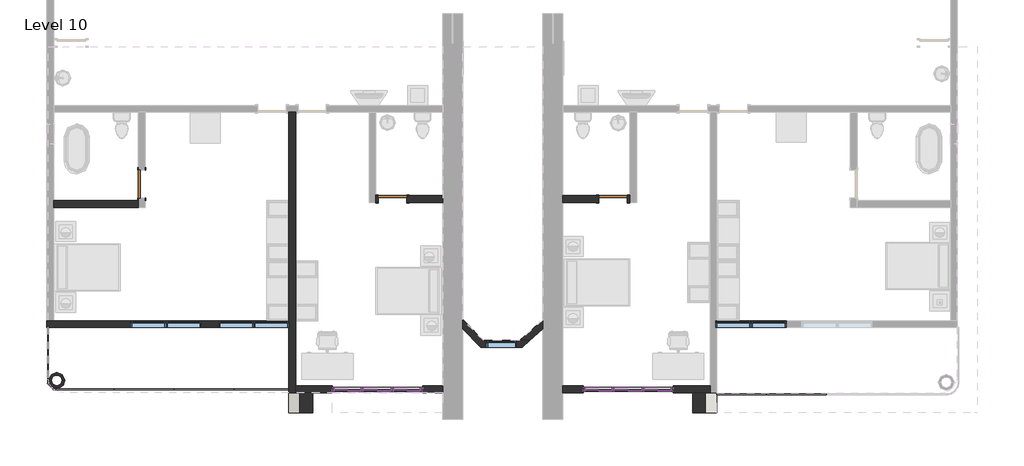
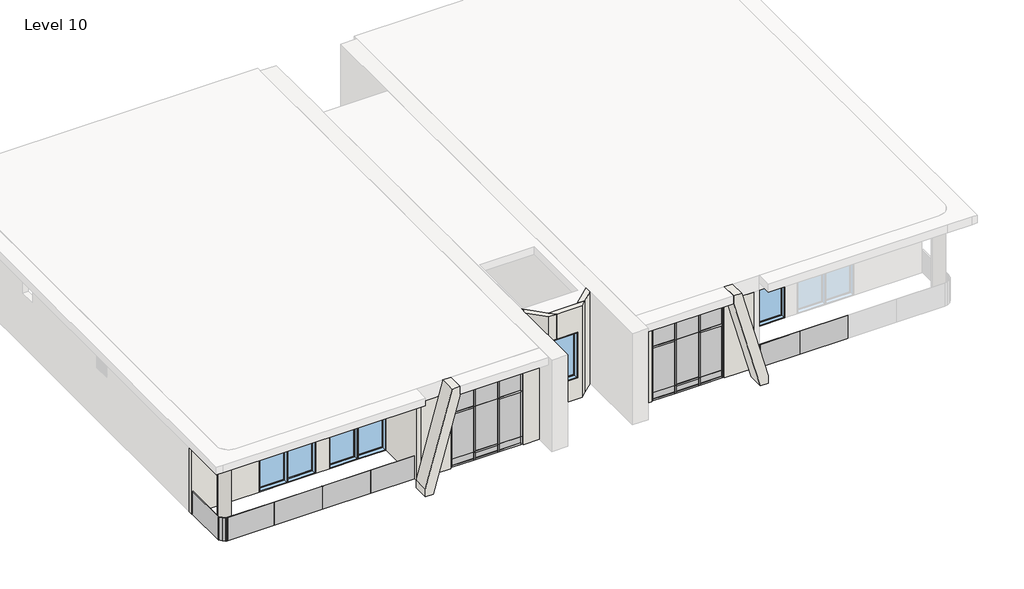
# One storey, part 1 of 3: 42 members, 29 plates, 16 walls, 7 windows, 3 doors.
"""IFC4 building model written with IfcOpenShell, lengths in millimetres."""

from ifc_helpers import new_model, si_unit, point, frame, frame_2d, origin, place, context, project, spatial, polyline, circle_curve, trimmed, segment, composite_curve, outline, extrude, faceted_brep, transform, mapped, element, save
from components import door_2703ae13, door_10fd3a06, member_c17f1be2, member_ad567e07, member_d2e7e466, member_7db1855a, member_75d1e245, member_d60e8053, member_3c3dc66a, member_2fae0574, member_410c6227, member_73c23c35, system_panel_glazed_38d54ecf, system_panel_glazed_fbb6c980, system_panel_glazed_4137532c, system_panel_glazed_6230de04, system_panel_glazed_a79f7f85, system_panel_glazed_9a5ea490, system_panel_glazed_95be5de7, system_panel_glazed_ffe51582, system_panel_glazed_8f95e3f6, system_panel_glazed_836907cd, system_panel_glazed_688a65a2, system_panel_glazed_c1a1c740, system_panel_glazed_22bcd51f, system_panel_glazed_524f965d, window_9a779fa2, window_1a213a25

model = new_model("IFC4")

# Units and contexts
model_context = context("Model", 3, world=origin())
ifc_project = project(units=[si_unit("LENGTHUNIT", "METRE", prefix="MILLI")], contexts=[model_context])

# Site, building, storey
site = spatial("IfcSite", under=ifc_project)
building = spatial("IfcBuilding", under=site)
storey = spatial("IfcBuildingStorey", under=building, Name="Level 10", Elevation=32918.4)

# Doors
placement = place(None, origin())
door_shape = door_2703ae13(model_context)
element("IfcDoor", 1, ObjectType="Door-Single-Panel.0001 : 34\" x 80\"", at=placement, inside=storey, context=model_context, shape_type="MappedRepresentation", body=[
    mapped(door_shape, transform((-15765.9987704, -441.9241442, 32918.4), x_axis=(0.0, -1.0, 0.0), y_axis=(1.0, 0.0, 0.0), z_axis=(0.0, 0.0, 1.0))),
])
element("IfcDoor", 2, ObjectType="Door-Single-Panel.0001 : 34\" x 80\"", at=placement, inside=storey, context=model_context, shape_type="MappedRepresentation", body=[
    mapped(door_shape, transform((-8145.9987704, -899.1241442, 32918.4), x_axis=(-1.0, 0.0, 0.0), y_axis=(0.0, -1.0, 0.0), z_axis=(0.0, 0.0, 1.0))),
])
door_2_shape = door_10fd3a06(model_context)
element("IfcDoor", 3, ObjectType="Door-Single-Panel.0001 : 34\" x 80\"", at=placement, inside=storey, context=model_context, shape_type="MappedRepresentation", body=[
    mapped(door_2_shape, transform((-1440.3987704, -899.1241442, 32918.4), x_axis=(1.0, 0.0, 0.0), y_axis=(0.0, 1.0, 0.0), z_axis=(0.0, 0.0, 1.0))),
])

# Members
member_shape = member_c17f1be2(model_context)
element("IfcMember", 4, ObjectType="Rectangular Mullion : 2.5\" x 5\" rectangular", at=placement, inside=storey, context=model_context, shape_type="MappedRepresentation", body=[
    mapped(member_shape, transform((-9911.2987704, -6690.3241442, 35966.4), x_axis=(0.0, 0.0, 1.0), y_axis=(0.0, 1.0, 0.0), z_axis=(-1.0, 0.0, 0.0))),
])
element("IfcMember", 5, ObjectType="Rectangular Mullion : 2.5\" x 5\" rectangular", at=placement, inside=storey, context=model_context, shape_type="MappedRepresentation", body=[
    mapped(member_shape, transform((-8114.2487704, -6690.3241442, 35966.4), x_axis=(0.0, 0.0, 1.0), y_axis=(0.0, 1.0, 0.0), z_axis=(-1.0, 0.0, 0.0))),
])
element("IfcMember", 6, ObjectType="Rectangular Mullion : 2.5\" x 5\" rectangular", at=placement, inside=storey, context=model_context, shape_type="MappedRepresentation", body=[
    mapped(member_shape, transform((-2291.2987704, -6690.3241442, 35966.4), x_axis=(0.0, 0.0, 1.0), y_axis=(0.0, 1.0, 0.0), z_axis=(-1.0, 0.0, 0.0))),
])
element("IfcMember", 7, ObjectType="Rectangular Mullion : 2.5\" x 5\" rectangular", at=placement, inside=storey, context=model_context, shape_type="MappedRepresentation", body=[
    mapped(member_shape, transform((-494.2487704, -6690.3241442, 35966.4), x_axis=(0.0, 0.0, 1.0), y_axis=(0.0, 1.0, 0.0), z_axis=(-1.0, 0.0, 0.0))),
])
element("IfcMember", 8, ObjectType="Rectangular Mullion : 2.5\" x 5\" rectangular", at=placement, inside=storey, context=model_context, shape_type="MappedRepresentation", body=[
    mapped(member_shape, transform((-7295.0987704, -6690.3241442, 32918.4), x_axis=(0.0, 0.0, -1.0), y_axis=(0.0, 1.0, 0.0), z_axis=(1.0, 0.0, 0.0))),
])
element("IfcMember", 9, ObjectType="Rectangular Mullion : 2.5\" x 5\" rectangular", at=placement, inside=storey, context=model_context, shape_type="MappedRepresentation", body=[
    mapped(member_shape, transform((-9092.1487704, -6690.3241442, 32918.4), x_axis=(0.0, 0.0, -1.0), y_axis=(0.0, 1.0, 0.0), z_axis=(1.0, 0.0, 0.0))),
])
element("IfcMember", 10, ObjectType="Rectangular Mullion : 2.5\" x 5\" rectangular", at=placement, inside=storey, context=model_context, shape_type="MappedRepresentation", body=[
    mapped(member_shape, transform((324.9012296, -6690.3241442, 32918.4), x_axis=(0.0, 0.0, -1.0), y_axis=(0.0, 1.0, 0.0), z_axis=(1.0, 0.0, 0.0))),
])
element("IfcMember", 11, ObjectType="Rectangular Mullion : 2.5\" x 5\" rectangular", at=placement, inside=storey, context=model_context, shape_type="MappedRepresentation", body=[
    mapped(member_shape, transform((-1472.1487704, -6690.3241442, 32918.4), x_axis=(0.0, 0.0, -1.0), y_axis=(0.0, 1.0, 0.0), z_axis=(1.0, 0.0, 0.0))),
])
member_2_shape = member_ad567e07(model_context)
element("IfcMember", 12, ObjectType="Rectangular Mullion : 2.5\" x 5\" rectangular", at=placement, inside=storey, context=model_context, shape_type="MappedRepresentation", body=[
    mapped(member_2_shape, transform((-8114.2487704, -6690.3241442, 35052.0), x_axis=(0.0, 0.0, 1.0), y_axis=(0.0, 1.0, 0.0), z_axis=(-1.0, 0.0, 0.0))),
])
element("IfcMember", 13, ObjectType="Rectangular Mullion : 2.5\" x 5\" rectangular", at=placement, inside=storey, context=model_context, shape_type="MappedRepresentation", body=[
    mapped(member_2_shape, transform((-9911.2987704, -6690.3241442, 35052.0), x_axis=(0.0, 0.0, 1.0), y_axis=(0.0, 1.0, 0.0), z_axis=(-1.0, 0.0, 0.0))),
])
element("IfcMember", 14, ObjectType="Rectangular Mullion : 2.5\" x 5\" rectangular", at=placement, inside=storey, context=model_context, shape_type="MappedRepresentation", body=[
    mapped(member_2_shape, transform((-494.2487704, -6690.3241442, 35052.0), x_axis=(0.0, 0.0, 1.0), y_axis=(0.0, 1.0, 0.0), z_axis=(-1.0, 0.0, 0.0))),
])
element("IfcMember", 15, ObjectType="Rectangular Mullion : 2.5\" x 5\" rectangular", at=placement, inside=storey, context=model_context, shape_type="MappedRepresentation", body=[
    mapped(member_2_shape, transform((-2291.2987704, -6690.3241442, 35052.0), x_axis=(0.0, 0.0, 1.0), y_axis=(0.0, 1.0, 0.0), z_axis=(-1.0, 0.0, 0.0))),
])
member_3_shape = member_d2e7e466(model_context)
element("IfcMember", 16, ObjectType="Rectangular Mullion : 2.5\" x 5\" rectangular", at=placement, inside=storey, context=model_context, shape_type="MappedRepresentation", body=[
    mapped(member_3_shape, transform((-8177.7487704, -6690.3241442, 32918.4), x_axis=(0.0, 0.0, -1.0), y_axis=(0.0, 1.0, 0.0), z_axis=(1.0, 0.0, 0.0))),
])
element("IfcMember", 17, ObjectType="Rectangular Mullion : 2.5\" x 5\" rectangular", at=placement, inside=storey, context=model_context, shape_type="MappedRepresentation", body=[
    mapped(member_3_shape, transform((-557.7487704, -6690.3241442, 32918.4), x_axis=(0.0, 0.0, -1.0), y_axis=(0.0, 1.0, 0.0), z_axis=(1.0, 0.0, 0.0))),
])
member_4_shape = member_7db1855a(model_context)
element("IfcMember", 18, ObjectType="Rectangular Mullion : 2.5\" x 5\" rectangular", at=placement, inside=storey, context=model_context, shape_type="MappedRepresentation", body=[
    mapped(member_4_shape, transform((-9028.6487704, -6690.3241442, 33223.2), x_axis=(0.0, 0.0, 1.0), y_axis=(0.0, 1.0, 0.0), z_axis=(-1.0, 0.0, 0.0))),
])
element("IfcMember", 19, ObjectType="Rectangular Mullion : 2.5\" x 5\" rectangular", at=placement, inside=storey, context=model_context, shape_type="MappedRepresentation", body=[
    mapped(member_4_shape, transform((-1408.6487704, -6690.3241442, 33223.2), x_axis=(0.0, 0.0, 1.0), y_axis=(0.0, 1.0, 0.0), z_axis=(-1.0, 0.0, 0.0))),
])
element("IfcMember", 20, ObjectType="Rectangular Mullion : 2.5\" x 5\" rectangular", at=placement, inside=storey, context=model_context, shape_type="MappedRepresentation", body=[
    mapped(member_3_shape, transform((-9028.6487704, -6690.3241442, 35966.4), x_axis=(0.0, 0.0, 1.0), y_axis=(0.0, 1.0, 0.0), z_axis=(-1.0, 0.0, 0.0))),
])
element("IfcMember", 21, ObjectType="Rectangular Mullion : 2.5\" x 5\" rectangular", at=placement, inside=storey, context=model_context, shape_type="MappedRepresentation", body=[
    mapped(member_3_shape, transform((-1408.6487704, -6690.3241442, 35966.4), x_axis=(0.0, 0.0, 1.0), y_axis=(0.0, 1.0, 0.0), z_axis=(-1.0, 0.0, 0.0))),
])
member_5_shape = member_75d1e245(model_context)
element("IfcMember", 22, ObjectType="Rectangular Mullion : 2.5\" x 5\" rectangular", at=placement, inside=storey, context=model_context, shape_type="MappedRepresentation", body=[
    mapped(member_5_shape, transform((-8145.9987704, -6690.3241442, 32918.4), x_axis=(-1.0, 0.0, 0.0), y_axis=(0.0, 1.0, 0.0), z_axis=(0.0, 0.0, -1.0))),
])
element("IfcMember", 23, ObjectType="Rectangular Mullion : 2.5\" x 5\" rectangular", at=placement, inside=storey, context=model_context, shape_type="MappedRepresentation", body=[
    mapped(member_5_shape, transform((-9060.3987704, -6690.3241442, 32918.4), x_axis=(-1.0, 0.0, 0.0), y_axis=(0.0, 1.0, 0.0), z_axis=(0.0, 0.0, -1.0))),
])
element("IfcMember", 24, ObjectType="Rectangular Mullion : 2.5\" x 5\" rectangular", at=placement, inside=storey, context=model_context, shape_type="MappedRepresentation", body=[
    mapped(member_5_shape, transform((-525.9987704, -6690.3241442, 32918.4), x_axis=(-1.0, 0.0, 0.0), y_axis=(0.0, 1.0, 0.0), z_axis=(0.0, 0.0, -1.0))),
])
element("IfcMember", 25, ObjectType="Rectangular Mullion : 2.5\" x 5\" rectangular", at=placement, inside=storey, context=model_context, shape_type="MappedRepresentation", body=[
    mapped(member_5_shape, transform((-1440.3987704, -6690.3241442, 32918.4), x_axis=(-1.0, 0.0, 0.0), y_axis=(0.0, 1.0, 0.0), z_axis=(0.0, 0.0, -1.0))),
])
member_6_shape = member_d60e8053(model_context)
element("IfcMember", 26, ObjectType="Rectangular Mullion : 2.5\" x 5\" rectangular", at=placement, inside=storey, context=model_context, shape_type="MappedRepresentation", body=[
    mapped(member_6_shape, transform((-8145.9987704, -6690.3241442, 33223.2), x_axis=(-1.0, 0.0, 0.0), y_axis=(0.0, 1.0, 0.0), z_axis=(0.0, 0.0, -1.0))),
])
element("IfcMember", 27, ObjectType="Rectangular Mullion : 2.5\" x 5\" rectangular", at=placement, inside=storey, context=model_context, shape_type="MappedRepresentation", body=[
    mapped(member_6_shape, transform((-9060.3987704, -6690.3241442, 33223.2), x_axis=(-1.0, 0.0, 0.0), y_axis=(0.0, 1.0, 0.0), z_axis=(0.0, 0.0, -1.0))),
])
element("IfcMember", 28, ObjectType="Rectangular Mullion : 2.5\" x 5\" rectangular", at=placement, inside=storey, context=model_context, shape_type="MappedRepresentation", body=[
    mapped(member_6_shape, transform((-525.9987704, -6690.3241442, 33223.2), x_axis=(-1.0, 0.0, 0.0), y_axis=(0.0, 1.0, 0.0), z_axis=(0.0, 0.0, -1.0))),
])
element("IfcMember", 29, ObjectType="Rectangular Mullion : 2.5\" x 5\" rectangular", at=placement, inside=storey, context=model_context, shape_type="MappedRepresentation", body=[
    mapped(member_6_shape, transform((-1440.3987704, -6690.3241442, 33223.2), x_axis=(-1.0, 0.0, 0.0), y_axis=(0.0, 1.0, 0.0), z_axis=(0.0, 0.0, -1.0))),
])
member_7_shape = member_3c3dc66a(model_context)
element("IfcMember", 30, ObjectType="Rectangular Mullion : 2.5\" x 5\" rectangular", at=placement, inside=storey, context=model_context, shape_type="MappedRepresentation", body=[
    mapped(member_7_shape, transform((-9974.7987704, -6690.3241442, 32918.4), x_axis=(-1.0, 0.0, 0.0), y_axis=(0.0, 1.0, 0.0), z_axis=(0.0, 0.0, -1.0))),
])
element("IfcMember", 31, ObjectType="Rectangular Mullion : 2.5\" x 5\" rectangular", at=placement, inside=storey, context=model_context, shape_type="MappedRepresentation", body=[
    mapped(member_7_shape, transform((-2354.7987704, -6690.3241442, 32918.4), x_axis=(-1.0, 0.0, 0.0), y_axis=(0.0, 1.0, 0.0), z_axis=(0.0, 0.0, -1.0))),
])
member_8_shape = member_2fae0574(model_context)
element("IfcMember", 32, ObjectType="Rectangular Mullion : 2.5\" x 5\" rectangular", at=placement, inside=storey, context=model_context, shape_type="MappedRepresentation", body=[
    mapped(member_8_shape, transform((-9974.7987704, -6690.3241442, 33223.2), x_axis=(-1.0, 0.0, 0.0), y_axis=(0.0, 1.0, 0.0), z_axis=(0.0, 0.0, -1.0))),
])
element("IfcMember", 33, ObjectType="Rectangular Mullion : 2.5\" x 5\" rectangular", at=placement, inside=storey, context=model_context, shape_type="MappedRepresentation", body=[
    mapped(member_8_shape, transform((-2354.7987704, -6690.3241442, 33223.2), x_axis=(-1.0, 0.0, 0.0), y_axis=(0.0, 1.0, 0.0), z_axis=(0.0, 0.0, -1.0))),
])
element("IfcMember", 34, ObjectType="Rectangular Mullion : 2.5\" x 5\" rectangular", at=placement, inside=storey, context=model_context, shape_type="MappedRepresentation", body=[
    mapped(member_8_shape, transform((-7231.5987704, -6690.3241442, 35052.0), x_axis=(1.0, 0.0, 0.0), y_axis=(0.0, 1.0, 0.0), z_axis=(0.0, 0.0, 1.0))),
])
element("IfcMember", 35, ObjectType="Rectangular Mullion : 2.5\" x 5\" rectangular", at=placement, inside=storey, context=model_context, shape_type="MappedRepresentation", body=[
    mapped(member_8_shape, transform((388.4012296, -6690.3241442, 35052.0), x_axis=(1.0, 0.0, 0.0), y_axis=(0.0, 1.0, 0.0), z_axis=(0.0, 0.0, 1.0))),
])
element("IfcMember", 36, ObjectType="Rectangular Mullion : 2.5\" x 5\" rectangular", at=placement, inside=storey, context=model_context, shape_type="MappedRepresentation", body=[
    mapped(member_7_shape, transform((-7231.5987704, -6690.3241442, 33223.2), x_axis=(1.0, 0.0, 0.0), y_axis=(0.0, 1.0, 0.0), z_axis=(0.0, 0.0, 1.0))),
])
element("IfcMember", 37, ObjectType="Rectangular Mullion : 2.5\" x 5\" rectangular", at=placement, inside=storey, context=model_context, shape_type="MappedRepresentation", body=[
    mapped(member_7_shape, transform((388.4012296, -6690.3241442, 33223.2), x_axis=(1.0, 0.0, 0.0), y_axis=(0.0, 1.0, 0.0), z_axis=(0.0, 0.0, 1.0))),
])
member_9_shape = member_410c6227(model_context)
element("IfcMember", 38, ObjectType="Rectangular Mullion : 2.5\" x 5\" rectangular", at=placement, inside=storey, context=model_context, shape_type="MappedRepresentation", body=[
    mapped(member_9_shape, transform((-8145.9987704, -6690.3241442, 35052.0), x_axis=(-1.0, 0.0, 0.0), y_axis=(0.0, 1.0, 0.0), z_axis=(0.0, 0.0, -1.0))),
])
element("IfcMember", 39, ObjectType="Rectangular Mullion : 2.5\" x 5\" rectangular", at=placement, inside=storey, context=model_context, shape_type="MappedRepresentation", body=[
    mapped(member_9_shape, transform((-9060.3987704, -6690.3241442, 35052.0), x_axis=(-1.0, 0.0, 0.0), y_axis=(0.0, 1.0, 0.0), z_axis=(0.0, 0.0, -1.0))),
])
element("IfcMember", 40, ObjectType="Rectangular Mullion : 2.5\" x 5\" rectangular", at=placement, inside=storey, context=model_context, shape_type="MappedRepresentation", body=[
    mapped(member_9_shape, transform((-525.9987704, -6690.3241442, 35052.0), x_axis=(-1.0, 0.0, 0.0), y_axis=(0.0, 1.0, 0.0), z_axis=(0.0, 0.0, -1.0))),
])
element("IfcMember", 41, ObjectType="Rectangular Mullion : 2.5\" x 5\" rectangular", at=placement, inside=storey, context=model_context, shape_type="MappedRepresentation", body=[
    mapped(member_9_shape, transform((-1440.3987704, -6690.3241442, 35052.0), x_axis=(-1.0, 0.0, 0.0), y_axis=(0.0, 1.0, 0.0), z_axis=(0.0, 0.0, -1.0))),
])
member_10_shape = member_73c23c35(model_context)
element("IfcMember", 42, ObjectType="Rectangular Mullion : 2.5\" x 5\" rectangular", at=placement, inside=storey, context=model_context, shape_type="MappedRepresentation", body=[
    mapped(member_10_shape, transform((-7231.5987704, -6690.3241442, 35966.4), x_axis=(1.0, 0.0, 0.0), y_axis=(0.0, 1.0, 0.0), z_axis=(0.0, 0.0, 1.0))),
])
element("IfcMember", 43, ObjectType="Rectangular Mullion : 2.5\" x 5\" rectangular", at=placement, inside=storey, context=model_context, shape_type="MappedRepresentation", body=[
    mapped(member_10_shape, transform((388.4012296, -6690.3241442, 35966.4), x_axis=(1.0, 0.0, 0.0), y_axis=(0.0, 1.0, 0.0), z_axis=(0.0, 0.0, 1.0))),
])
element("IfcMember", 44, ObjectType="Rectangular Mullion : 2.5\" x 5\" rectangular", at=placement, inside=storey, context=model_context, shape_type="MappedRepresentation", body=[
    mapped(member_10_shape, transform((-9974.7987704, -6690.3241442, 35052.0), x_axis=(-1.0, 0.0, 0.0), y_axis=(0.0, 1.0, 0.0), z_axis=(0.0, 0.0, -1.0))),
])
element("IfcMember", 45, ObjectType="Rectangular Mullion : 2.5\" x 5\" rectangular", at=placement, inside=storey, context=model_context, shape_type="MappedRepresentation", body=[
    mapped(member_10_shape, transform((-2354.7987704, -6690.3241442, 35052.0), x_axis=(-1.0, 0.0, 0.0), y_axis=(0.0, 1.0, 0.0), z_axis=(0.0, 0.0, -1.0))),
])

# Plates
system_panel_glazed_shape = system_panel_glazed_38d54ecf(model_context)
element("IfcPlate", 46, ObjectType="System Panel : Glazed", at=placement, inside=storey, context=model_context, shape_type="MappedRepresentation", body=[
    mapped(system_panel_glazed_shape, transform((-8603.1987704, -6690.3241442, 33254.95), x_axis=(-1.0, 0.0, 0.0), y_axis=(0.0, -1.0, 0.0), z_axis=(0.0, 0.0, 1.0))),
])
element("IfcPlate", 47, ObjectType="System Panel : Glazed", at=placement, inside=storey, context=model_context, shape_type="MappedRepresentation", body=[
    mapped(system_panel_glazed_shape, transform((-983.1987704, -6690.3241442, 33254.95), x_axis=(-1.0, 0.0, 0.0), y_axis=(0.0, -1.0, 0.0), z_axis=(0.0, 0.0, 1.0))),
])
system_panel_glazed_2_shape = system_panel_glazed_fbb6c980(model_context)
element("IfcPlate", 48, ObjectType="System Panel : Glazed", at=placement, inside=storey, context=model_context, shape_type="MappedRepresentation", body=[
    mapped(system_panel_glazed_2_shape, transform((-8603.1987704, -6690.3241442, 32981.9), x_axis=(-1.0, 0.0, 0.0), y_axis=(0.0, -1.0, 0.0), z_axis=(0.0, 0.0, 1.0))),
])
element("IfcPlate", 49, ObjectType="System Panel : Glazed", at=placement, inside=storey, context=model_context, shape_type="MappedRepresentation", body=[
    mapped(system_panel_glazed_2_shape, transform((-983.1987704, -6690.3241442, 32981.9), x_axis=(-1.0, 0.0, 0.0), y_axis=(0.0, -1.0, 0.0), z_axis=(0.0, 0.0, 1.0))),
])
system_panel_glazed_3_shape = system_panel_glazed_4137532c(model_context)
element("IfcPlate", 50, ObjectType="System Panel : Glazed", at=placement, inside=storey, context=model_context, shape_type="MappedRepresentation", body=[
    mapped(system_panel_glazed_3_shape, transform((-7704.6737704, -6690.3241442, 32981.9), x_axis=(-1.0, 0.0, 0.0), y_axis=(0.0, -1.0, 0.0), z_axis=(0.0, 0.0, 1.0))),
])
element("IfcPlate", 51, ObjectType="System Panel : Glazed", at=placement, inside=storey, context=model_context, shape_type="MappedRepresentation", body=[
    mapped(system_panel_glazed_3_shape, transform((-9501.7237704, -6690.3241442, 32981.9), x_axis=(-1.0, 0.0, 0.0), y_axis=(0.0, -1.0, 0.0), z_axis=(0.0, 0.0, 1.0))),
])
element("IfcPlate", 52, ObjectType="System Panel : Glazed", at=placement, inside=storey, context=model_context, shape_type="MappedRepresentation", body=[
    mapped(system_panel_glazed_3_shape, transform((-84.6737704, -6690.3241442, 32981.9), x_axis=(-1.0, 0.0, 0.0), y_axis=(0.0, -1.0, 0.0), z_axis=(0.0, 0.0, 1.0))),
])
element("IfcPlate", 53, ObjectType="System Panel : Glazed", at=placement, inside=storey, context=model_context, shape_type="MappedRepresentation", body=[
    mapped(system_panel_glazed_3_shape, transform((-1881.7237704, -6690.3241442, 32981.9), x_axis=(-1.0, 0.0, 0.0), y_axis=(0.0, -1.0, 0.0), z_axis=(0.0, 0.0, 1.0))),
])
system_panel_glazed_4_shape = system_panel_glazed_6230de04(model_context)
element("IfcPlate", 54, ObjectType="System Panel : Glazed", at=placement, inside=storey, context=model_context, shape_type="MappedRepresentation", body=[
    mapped(system_panel_glazed_4_shape, transform((-7704.6737704, -6690.3241442, 33223.2), x_axis=(-1.0, 0.0, 0.0), y_axis=(0.0, -1.0, 0.0), z_axis=(0.0, 0.0, 1.0))),
])
element("IfcPlate", 55, ObjectType="System Panel : Glazed", at=placement, inside=storey, context=model_context, shape_type="MappedRepresentation", body=[
    mapped(system_panel_glazed_4_shape, transform((-9501.7237704, -6690.3241442, 33223.2), x_axis=(-1.0, 0.0, 0.0), y_axis=(0.0, -1.0, 0.0), z_axis=(0.0, 0.0, 1.0))),
])
element("IfcPlate", 56, ObjectType="System Panel : Glazed", at=placement, inside=storey, context=model_context, shape_type="MappedRepresentation", body=[
    mapped(system_panel_glazed_4_shape, transform((-84.6737704, -6690.3241442, 33223.2), x_axis=(-1.0, 0.0, 0.0), y_axis=(0.0, -1.0, 0.0), z_axis=(0.0, 0.0, 1.0))),
])
element("IfcPlate", 57, ObjectType="System Panel : Glazed", at=placement, inside=storey, context=model_context, shape_type="MappedRepresentation", body=[
    mapped(system_panel_glazed_4_shape, transform((-1881.7237704, -6690.3241442, 33223.2), x_axis=(-1.0, 0.0, 0.0), y_axis=(0.0, -1.0, 0.0), z_axis=(0.0, 0.0, 1.0))),
])
system_panel_glazed_5_shape = system_panel_glazed_a79f7f85(model_context)
element("IfcPlate", 58, ObjectType="System Panel : Glazed", at=placement, inside=storey, context=model_context, shape_type="MappedRepresentation", body=[
    mapped(system_panel_glazed_5_shape, transform((-7704.6737704, -6690.3241442, 35083.75), x_axis=(-1.0, 0.0, 0.0), y_axis=(0.0, -1.0, 0.0), z_axis=(0.0, 0.0, 1.0))),
])
element("IfcPlate", 59, ObjectType="System Panel : Glazed", at=placement, inside=storey, context=model_context, shape_type="MappedRepresentation", body=[
    mapped(system_panel_glazed_5_shape, transform((-9501.7237704, -6690.3241442, 35083.75), x_axis=(-1.0, 0.0, 0.0), y_axis=(0.0, -1.0, 0.0), z_axis=(0.0, 0.0, 1.0))),
])
element("IfcPlate", 60, ObjectType="System Panel : Glazed", at=placement, inside=storey, context=model_context, shape_type="MappedRepresentation", body=[
    mapped(system_panel_glazed_5_shape, transform((-84.6737704, -6690.3241442, 35083.75), x_axis=(-1.0, 0.0, 0.0), y_axis=(0.0, -1.0, 0.0), z_axis=(0.0, 0.0, 1.0))),
])
element("IfcPlate", 61, ObjectType="System Panel : Glazed", at=placement, inside=storey, context=model_context, shape_type="MappedRepresentation", body=[
    mapped(system_panel_glazed_5_shape, transform((-1881.7237704, -6690.3241442, 35083.75), x_axis=(-1.0, 0.0, 0.0), y_axis=(0.0, -1.0, 0.0), z_axis=(0.0, 0.0, 1.0))),
])
system_panel_glazed_6_shape = system_panel_glazed_9a5ea490(model_context)
element("IfcPlate", 62, ObjectType="System Panel : Glazed", at=placement, inside=storey, context=model_context, shape_type="MappedRepresentation", body=[
    mapped(system_panel_glazed_6_shape, transform((-8603.1987704, -6690.3241442, 35052.0), x_axis=(-1.0, 0.0, 0.0), y_axis=(0.0, -1.0, 0.0), z_axis=(0.0, 0.0, 1.0))),
])
element("IfcPlate", 63, ObjectType="System Panel : Glazed", at=placement, inside=storey, context=model_context, shape_type="MappedRepresentation", body=[
    mapped(system_panel_glazed_6_shape, transform((-983.1987704, -6690.3241442, 35052.0), x_axis=(-1.0, 0.0, 0.0), y_axis=(0.0, -1.0, 0.0), z_axis=(0.0, 0.0, 1.0))),
])
system_panel_glazed_7_shape = system_panel_glazed_95be5de7(model_context)
element("IfcPlate", 64, ObjectType="System Panel : Glazed", at=placement, inside=storey, context=model_context, shape_type="MappedRepresentation", body=[
    mapped(system_panel_glazed_7_shape, transform((-15707.2305745, -6723.6923401, 32918.4), x_axis=(1.0, 0.0, 0.0), y_axis=(0.0, 1.0, 0.0), z_axis=(0.0, 0.0, 1.0))),
])
element("IfcPlate", 65, ObjectType="System Panel : Glazed", at=placement, inside=storey, context=model_context, shape_type="MappedRepresentation", body=[
    mapped(system_panel_glazed_7_shape, transform((-13878.4305745, -6723.6923401, 32918.4), x_axis=(1.0, 0.0, 0.0), y_axis=(0.0, 1.0, 0.0), z_axis=(0.0, 0.0, 1.0))),
])
element("IfcPlate", 66, ObjectType="System Panel : Glazed", at=placement, inside=storey, context=model_context, shape_type="MappedRepresentation", body=[
    mapped(system_panel_glazed_7_shape, transform((4129.1120092, -6810.4133646, 32918.4), x_axis=(-1.0, 0.0, 0.0), y_axis=(0.0, -1.0, 0.0), z_axis=(0.0, 0.0, 1.0))),
])
system_panel_glazed_8_shape = system_panel_glazed_ffe51582(model_context)
element("IfcPlate", 67, ObjectType="System Panel : Glazed", at=placement, inside=storey, context=model_context, shape_type="MappedRepresentation", body=[
    mapped(system_panel_glazed_8_shape, transform((-18451.9713429, -6722.1515718, 32918.4), x_axis=(0.7071067811865462, -0.7071067811865488, 0.0), y_axis=(0.7071067811865488, 0.7071067811865462, 0.0), z_axis=(0.0, 0.0, 1.0))),
])
system_panel_glazed_9_shape = system_panel_glazed_8f95e3f6(model_context)
element("IfcPlate", 68, ObjectType="System Panel : Glazed", at=placement, inside=storey, context=model_context, shape_type="MappedRepresentation", body=[
    mapped(system_panel_glazed_9_shape, transform((-18648.8987704, -5667.9741442, 32918.4), x_axis=(0.0, -1.0, 0.0), y_axis=(1.0, 0.0, 0.0), z_axis=(0.0, 0.0, 1.0))),
])
system_panel_glazed_10_shape = system_panel_glazed_836907cd(model_context)
element("IfcPlate", 69, ObjectType="System Panel : Glazed", at=placement, inside=storey, context=model_context, shape_type="MappedRepresentation", body=[
    mapped(system_panel_glazed_10_shape, transform((-18418.6805745, -6723.6923401, 32918.4), x_axis=(1.0, 0.0, 0.0), y_axis=(0.0, 1.0, 0.0), z_axis=(0.0, 0.0, 1.0))),
])
system_panel_glazed_11_shape = system_panel_glazed_688a65a2(model_context)
element("IfcPlate", 70, ObjectType="System Panel : Glazed", at=placement, inside=storey, context=model_context, shape_type="MappedRepresentation", body=[
    mapped(system_panel_glazed_11_shape, transform((-12129.8146725, -6723.6923401, 32918.4), x_axis=(1.0, 0.0, 0.0), y_axis=(0.0, 1.0, 0.0), z_axis=(0.0, 0.0, 1.0))),
])
system_panel_glazed_12_shape = system_panel_glazed_c1a1c740(model_context)
element("IfcPlate", 71, ObjectType="System Panel : Glazed", at=placement, inside=storey, context=model_context, shape_type="MappedRepresentation", body=[
    mapped(system_panel_glazed_12_shape, transform((-17504.2805745, -6723.6923401, 32918.4), x_axis=(1.0, 0.0, 0.0), y_axis=(0.0, 1.0, 0.0), z_axis=(0.0, 0.0, 1.0))),
])
system_panel_glazed_13_shape = system_panel_glazed_22bcd51f(model_context)
element("IfcPlate", 72, ObjectType="System Panel : Glazed", at=placement, inside=storey, context=model_context, shape_type="MappedRepresentation", body=[
    mapped(system_panel_glazed_13_shape, transform((-18600.0521056, -6574.070809, 32918.4), x_axis=(0.7071067811865462, -0.7071067811865488, 0.0), y_axis=(0.7071067811865488, 0.7071067811865462, 0.0), z_axis=(0.0, 0.0, 1.0))),
])
element("IfcPlate", 73, ObjectType="System Panel : Glazed", at=placement, inside=storey, context=model_context, shape_type="MappedRepresentation", body=[
    mapped(system_panel_glazed_13_shape, transform((-18502.3587761, -6671.7641386, 32918.4), x_axis=(0.7071067811865462, -0.7071067811865488, 0.0), y_axis=(0.7071067811865488, 0.7071067811865462, 0.0), z_axis=(0.0, 0.0, 1.0))),
])
system_panel_glazed_14_shape = system_panel_glazed_524f965d(model_context)
element("IfcPlate", 74, ObjectType="System Panel : Glazed", at=placement, inside=storey, context=model_context, shape_type="MappedRepresentation", body=[
    mapped(system_panel_glazed_14_shape, transform((2461.6914958, -6810.4133646, 32918.4), x_axis=(-1.0, 0.0, 0.0), y_axis=(0.0, -1.0, 0.0), z_axis=(0.0, 0.0, 1.0))),
])

# Walls
element("IfcWall", 75, ObjectType="Generic - 3\" green 2", at=placement, inside=storey, context=model_context, shape_type="SweptSolid", body=[
    extrude(outline(composite_curve([segment(polyline([(-18518.7237704, -6418.8616442), (-18594.9237704, -6418.8616442)]), True, "CONTINUOUS"), segment(trimmed(circle_curve(frame_2d((-18353.6237704, -6418.8616442)), 241.3), [point((-18594.9237704, -6418.8616442))], [point((-18112.3237704, -6418.8616442))], False, "CARTESIAN"), True, "CONTINUOUS"), segment(polyline([(-18112.3237704, -6418.8616442), (-18188.5237704, -6418.8616442)]), True, "CONTINUOUS"), segment(trimmed(circle_curve(frame_2d((-18353.6237704, -6418.8616442)), 165.1), [point((-18188.5237704, -6418.8616442))], [point((-18518.7237704, -6418.8616442))], True, "CARTESIAN"), True, "CONTINUOUS")], self_intersect=False)), frame((0.0, 0.0, 32918.4), z_axis=(0.0, 0.0, 1.0), x_axis=(1.0, 0.0, 0.0)), (0.0, 0.0, 1.0), 3048.0),
])
element("IfcWall", 76, ObjectType="Generic - 3\" green 2", at=placement, inside=storey, context=model_context, shape_type="SweptSolid", body=[
    extrude(outline(composite_curve([segment(polyline([(-18188.5237704, -6418.8616442), (-18112.3237704, -6418.8616442)]), True, "CONTINUOUS"), segment(trimmed(circle_curve(frame_2d((-18353.6237704, -6418.8616442)), 241.3), [point((-18112.3237704, -6418.8616442))], [point((-18594.9237704, -6418.8616442))], False, "CARTESIAN"), True, "CONTINUOUS"), segment(polyline([(-18594.9237704, -6418.8616442), (-18518.7237704, -6418.8616442)]), True, "CONTINUOUS"), segment(trimmed(circle_curve(frame_2d((-18353.6237704, -6418.8616442)), 165.1), [point((-18518.7237704, -6418.8616442))], [point((-18188.5237704, -6418.8616442))], True, "CARTESIAN"), True, "CONTINUOUS")], self_intersect=False)), frame((0.0, 0.0, 32918.4), z_axis=(0.0, 0.0, 1.0), x_axis=(1.0, 0.0, 0.0)), (0.0, 0.0, 1.0), 3048.0),
])
element("IfcWall", 77, ObjectType="Generic - 8\" cream", at=placement, inside=storey, context=model_context, shape_type="Brep", body=[
    faceted_brep([(-11295.5987704, 1742.4758558, 32918.4), (-11295.5987704, -6791.9241442, 32918.4), (-11295.5987704, -6791.9241442, 35966.4), (-11295.5987704, -4810.7241442, 35966.4), (-11295.5987704, -4607.5241442, 35966.4), (-11295.5987704, 1742.4758558, 35966.4), (-11092.3987704, 1742.4758558, 32918.4), (-11092.3987704, 1742.4758558, 35966.4), (-11092.3987704, -6588.7241442, 35966.4), (-11092.3987704, -6791.9241442, 35966.4), (-11092.3987704, -6791.9241442, 32918.4), (-11092.3987704, -6588.7241442, 32918.4)], [[[0, 1, 2, 3, 4, 5]], [[6, 7, 8, 9, 10, 11]], [[1, 0, 6, 11, 10]], [[5, 4, 3, 2, 9, 8, 7]], [[0, 5, 7, 6]], [[2, 1, 10, 9]]]),
])
element("IfcWall", 78, ObjectType="Generic - 8\" cream", at=placement, inside=storey, context=model_context, shape_type="SweptSolid", body=[
    extrude(outline(polyline([(-18445.6987704, -949.9241442), (-15867.5987704, -949.9241442), (-15867.5987704, -1153.1241442), (-18445.6987704, -1153.1241442), (-18445.6987704, -949.9241442)])), frame((0.0, 0.0, 32918.4), z_axis=(0.0, 0.0, 1.0), x_axis=(1.0, 0.0, 0.0)), (0.0, 0.0, 1.0), 3048.0),
])
element("IfcWall", 79, ObjectType="Generic - 8\" cream", at=placement, inside=storey, context=model_context, shape_type="SweptSolid", body=[
    extrude(outline(polyline([(35966.4, -6621.9987704), (35966.4, -8653.9987704), (32918.4, -8653.9987704), (32918.4, -8577.7987704), (34950.4, -8577.7987704), (34950.4, -7714.1987704), (32918.4, -7714.1987704), (32918.4, -6621.9987704), (35966.4, -6621.9987704)])), frame((0.0, -1000.7241442, 0.0), z_axis=(0.0, 1.0, 0.0), x_axis=(0.0, 0.0, 1.0)), (0.0, 0.0, 1.0), 203.2),
])
element("IfcWall", 80, ObjectType="Generic - 8\" cream", at=placement, inside=storey, context=model_context, shape_type="Brep", body=[
    faceted_brep([(-18648.8987704, -4607.5241442, 35966.4), (-18445.6987704, -4607.5241442, 35966.4), (-11295.5987704, -4607.5241442, 35966.4), (-11295.5987704, -4607.5241442, 35661.6), (-13429.1987704, -4607.5241442, 35661.6), (-13429.1987704, -4607.5241442, 32918.4), (-13962.5987704, -4607.5241442, 32918.4), (-13962.5987704, -4607.5241442, 35661.6), (-16096.1987704, -4607.5241442, 35661.6), (-16096.1987704, -4607.5241442, 32918.4), (-18445.6987704, -4607.5241442, 32918.4), (-18648.8987704, -4607.5241442, 32918.4), (-11295.5987704, -4810.7241442, 35966.4), (-18648.8987704, -4810.7241442, 35966.4), (-18648.8987704, -4810.7241442, 32918.4), (-16096.1987704, -4810.7241442, 32918.4), (-16096.1987704, -4810.7241442, 35661.6), (-13962.5987704, -4810.7241442, 35661.6), (-13962.5987704, -4810.7241442, 32918.4), (-13429.1987704, -4810.7241442, 32918.4), (-13429.1987704, -4810.7241442, 35661.6), (-11295.5987704, -4810.7241442, 35661.6)], [[[0, 1, 2, 3, 4, 5, 6, 7, 8, 9, 10, 11]], [[12, 13, 14, 15, 16, 17, 18, 19, 20, 21]], [[14, 11, 10, 9, 15]], [[5, 19, 18, 6]], [[2, 1, 0, 13, 12]], [[2, 12, 21, 3]], [[0, 11, 14, 13]], [[3, 21, 20, 4]], [[4, 20, 19, 5]], [[17, 7, 6, 18]], [[7, 17, 16, 8]], [[8, 16, 15, 9]]]),
])
element("IfcWall", 81, ObjectType="Generic - 8\" cream", at=placement, inside=storey, context=model_context, shape_type="SweptSolid", body=[
    extrude(outline(polyline([(35966.4, -932.3987704), (35966.4, -2964.3987704), (32918.4, -2964.3987704), (32918.4, -1872.1987704), (34950.4, -1872.1987704), (34950.4, -1008.5987704), (32918.4, -1008.5987704), (32918.4, -932.3987704), (35966.4, -932.3987704)])), frame((0.0, -1000.7241442, 0.0), z_axis=(0.0, 1.0, 0.0), x_axis=(0.0, 0.0, 1.0)), (0.0, 0.0, 1.0), 203.2),
])
element("IfcWall", 82, ObjectType="Generic - 8\" cream", at=placement, inside=storey, context=model_context, shape_type="SweptSolid", body=[
    extrude(outline(polyline([(388.4012296, -6588.7241442), (1506.0012296, -6588.7241442), (1506.0012296, -6791.9241442), (388.4012296, -6791.9241442), (388.4012296, -6588.7241442)])), frame((0.0, 0.0, 32918.4), z_axis=(0.0, 0.0, 1.0), x_axis=(1.0, 0.0, 0.0)), (0.0, 0.0, 1.0), 3048.0),
])
element("IfcWall", 83, ObjectType="Generic - 8\" cream", at=placement, inside=storey, context=model_context, shape_type="SweptSolid", body=[
    extrude(outline(polyline([(-2354.7987704, -6791.9241442), (-2964.3987704, -6791.9241442), (-2964.3987704, -6588.7241442), (-2354.7987704, -6588.7241442), (-2354.7987704, -6791.9241442)])), frame((0.0, 0.0, 32918.4), z_axis=(0.0, 0.0, 1.0), x_axis=(1.0, 0.0, 0.0)), (0.0, 0.0, 1.0), 3048.0),
])
element("IfcWall", 84, ObjectType="Generic - 8\" cream", at=placement, inside=storey, context=model_context, shape_type="SweptSolid", body=[
    extrude(outline(polyline([(-9974.7987704, -6791.9241442), (-11092.3987704, -6791.9241442), (-11092.3987704, -6588.7241442), (-9974.7987704, -6588.7241442), (-9974.7987704, -6791.9241442)])), frame((0.0, 0.0, 32918.4), z_axis=(0.0, 0.0, 1.0), x_axis=(1.0, 0.0, 0.0)), (0.0, 0.0, 1.0), 3048.0),
])
element("IfcWall", 85, ObjectType="Generic - 8\" cream", at=placement, inside=storey, context=model_context, shape_type="SweptSolid", body=[
    extrude(outline(polyline([(-7231.5987704, -6588.7241442), (-6621.9987704, -6588.7241442), (-6621.9987704, -6791.9241442), (-7231.5987704, -6791.9241442), (-7231.5987704, -6588.7241442)])), frame((0.0, 0.0, 32918.4), z_axis=(0.0, 0.0, 1.0), x_axis=(1.0, 0.0, 0.0)), (0.0, 0.0, 1.0), 3048.0),
])
element("IfcWall", 86, ObjectType="Generic - 8\" green", at=placement, inside=storey, context=model_context, shape_type="Brep", body=[
    faceted_brep([(-6012.3987704, -4852.8082422, 32918.4), (-5458.7044276, -5406.502585, 32918.4), (-5458.7044276, -5406.502585, 36576.0), (-6012.3987704, -4852.8082422, 36576.0), (-5171.3362318, -5406.502585, 32918.4), (-5374.5362318, -5203.302585, 32918.4), (-6012.3987704, -4565.4400463, 32918.4), (-6012.3987704, -4565.4400463, 36576.0), (-5374.5362318, -5203.302585, 36576.0), (-5171.3362318, -5406.502585, 36576.0), (-5171.3362318, -5406.502585, 35585.4), (-5289.4901401, -5288.3486766, 35585.4), (-5289.4901401, -5288.3486766, 33756.6), (-5171.3362318, -5406.502585, 33756.6), (-5289.4901401, -5406.502585, 33756.6), (-5289.4901401, -5406.502585, 35585.4)], [[[0, 1, 2, 3]], [[4, 5, 6, 7, 8, 9, 10, 11, 12, 13]], [[1, 0, 6, 5, 4]], [[3, 2, 9, 8, 7]], [[0, 3, 7, 6]], [[2, 1, 4, 13, 14, 15, 10, 9]], [[12, 14, 13]], [[14, 12, 11, 15]], [[15, 11, 10]]]),
])
element("IfcWall", 87, ObjectType="Generic - 8\" green", at=placement, inside=storey, context=model_context, shape_type="Brep", body=[
    faceted_brep([(-5171.3362318, -5406.502585, 32918.4), (-4203.3343712, -5406.502585, 32918.4), (-4203.3343712, -5406.502585, 36576.0), (-5171.3362318, -5406.502585, 36576.0), (-5171.3362318, -5406.502585, 35585.4), (-4375.0901401, -5406.502585, 35585.4), (-4375.0901401, -5406.502585, 33756.6), (-5171.3362318, -5406.502585, 33756.6), (-3975.4820774, -5203.302585, 32918.4), (-4280.7801413, -5203.302585, 32918.4), (-5374.5362318, -5203.302585, 32918.4), (-5374.5362318, -5203.302585, 36576.0), (-4280.7801413, -5203.302585, 36576.0), (-3975.4820774, -5203.302585, 36576.0), (-4375.0901401, -5203.302585, 33756.6), (-4375.0901401, -5203.302585, 35585.4), (-5289.4901401, -5203.302585, 35585.4), (-5289.4901401, -5203.302585, 33756.6), (-5289.4901401, -5288.3486766, 33756.6), (-5289.4901401, -5288.3486766, 35585.4)], [[[0, 1, 2, 3, 4, 5, 6, 7]], [[8, 9, 10, 11, 12, 13], [14, 15, 16, 17]], [[1, 0, 10, 9, 8]], [[3, 2, 13, 12, 11]], [[3, 11, 10, 0, 7, 18, 19, 4]], [[2, 1, 8, 13]], [[5, 15, 14, 6]], [[6, 14, 17, 18, 7]], [[18, 17, 16, 19]], [[15, 5, 4, 19, 16]]]),
])
element("IfcWall", 88, ObjectType="Generic - 8\" green", at=placement, inside=storey, context=model_context, shape_type="SweptSolid", body=[
    extrude(outline(polyline([(-3573.9987704, -4845.2574382), (-3975.4820774, -5203.302585), (-4280.7801413, -5203.302585), (-3573.9987704, -4572.9908503), (-3573.9987704, -4845.2574382)])), frame((0.0, 0.0, 32918.4), z_axis=(0.0, 0.0, 1.0), x_axis=(1.0, 0.0, 0.0)), (0.0, 0.0, 1.0), 3657.6),
])
element("IfcWall", 89, ObjectType="Generic -2' white 2", at=placement, inside=storey, context=model_context, shape_type="SweptSolid", body=[
    extrude(outline(polyline([(36271.2, -9974.7987704), (36576.0, -9974.7987704), (36576.0, -10279.5987704), (32918.4, -11295.5987704), (32613.6, -11295.5987704), (32613.6, -10990.7987704), (36271.2, -9974.7987704)])), frame((0.0, -7401.5241442, 0.0), z_axis=(0.0, 1.0, 0.0), x_axis=(0.0, 0.0, 1.0)), (0.0, 0.0, 1.0), 609.6),
])
element("IfcWall", 90, ObjectType="Generic -2' white 2", at=placement, inside=storey, context=model_context, shape_type="SweptSolid", body=[
    extrude(outline(polyline([(36271.2, 387.8709824), (32613.6, 1403.8709824), (32613.6, 1708.6709824), (32918.4, 1708.6709824), (36576.0, 692.6709824), (36576.0, 387.8709824), (36271.2, 387.8709824)])), frame((0.0, -7401.5241442, 0.0), z_axis=(0.0, 1.0, 0.0), x_axis=(0.0, 0.0, 1.0)), (0.0, 0.0, 1.0), 609.6),
])

# Windows
window_shape = window_9a779fa2(model_context)
element("IfcWindow", 91, ObjectType="Fixed : 36\" x 72\"", at=placement, inside=storey, context=model_context, shape_type="MappedRepresentation", body=[
    mapped(window_shape, transform((-4794.1901401, -5304.902585, 33451.8), x_axis=(1.0, 0.0, 0.0), y_axis=(0.0, 1.0, 0.0), z_axis=(0.0, 0.0, 1.0))),
])
window_2_shape = window_1a213a25(model_context)
element("IfcWindow", 92, ObjectType="Fixed : 36\" x 72\" 2", at=placement, inside=storey, context=model_context, shape_type="MappedRepresentation", body=[
    mapped(window_2_shape, transform((-11790.8987704, -4709.1241442, 32613.6), x_axis=(1.0, 0.0, 0.0), y_axis=(0.0, 1.0, 0.0), z_axis=(0.0, 0.0, 1.0))),
])
element("IfcWindow", 93, ObjectType="Fixed : 36\" x 72\" 2", at=placement, inside=storey, context=model_context, shape_type="MappedRepresentation", body=[
    mapped(window_2_shape, transform((-12857.6987704, -4709.1241442, 32613.6), x_axis=(1.0, 0.0, 0.0), y_axis=(0.0, 1.0, 0.0), z_axis=(0.0, 0.0, 1.0))),
])
element("IfcWindow", 94, ObjectType="Fixed : 36\" x 72\" 2", at=placement, inside=storey, context=model_context, shape_type="MappedRepresentation", body=[
    mapped(window_2_shape, transform((-14457.8987704, -4709.1241442, 32613.6), x_axis=(1.0, 0.0, 0.0), y_axis=(0.0, 1.0, 0.0), z_axis=(0.0, 0.0, 1.0))),
])
element("IfcWindow", 95, ObjectType="Fixed : 36\" x 72\" 2", at=placement, inside=storey, context=model_context, shape_type="MappedRepresentation", body=[
    mapped(window_2_shape, transform((-15524.6987704, -4709.1241442, 32613.6), x_axis=(1.0, 0.0, 0.0), y_axis=(0.0, 1.0, 0.0), z_axis=(0.0, 0.0, 1.0))),
])
element("IfcWindow", 96, ObjectType="Fixed : 36\" x 72\" 2", at=placement, inside=storey, context=model_context, shape_type="MappedRepresentation", body=[
    mapped(window_2_shape, transform((2255.3012296, -4709.1241442, 32613.6), x_axis=(1.0, 0.0, 0.0), y_axis=(0.0, 1.0, 0.0), z_axis=(0.0, 0.0, 1.0))),
])
element("IfcWindow", 97, ObjectType="Fixed : 36\" x 72\" 2", at=placement, inside=storey, context=model_context, shape_type="MappedRepresentation", body=[
    mapped(window_2_shape, transform((3331.6262296, -4709.1241442, 32613.6), x_axis=(1.0, 0.0, 0.0), y_axis=(0.0, 1.0, 0.0), z_axis=(0.0, 0.0, 1.0))),
])

save(model, "model.ifc")

# Revit data of these elements
# Type "Door-Single-Panel.0001 : 34\" x 80\""
#   Type Mark = "9"
#   Construction Type Id = "DOOR"
#   Assembly Code = "C1020300"
#   Analytic Construction = "Wooden"
#   Thickness = 0' - 2"
#   Thermal Resistance (R) = 0.455703 (m²·K)/W
#   Swing Angle [instance default] = 90.00°
#   Heat Transfer Coefficient (U) = 2.19465 W/(m²·K)
#   Height = 6' - 8"
#   Trim Projection Ext = 0' - 1"
#   Trim Projection Int = 0' - 1"
#   Trim Width = 0' - 3"
#   Width = 2' - 10"
#   Panel Material = Wood - Birch - Solid Stained Light Low Gloss
#   Trim Material = Paint - Sienna
#   Visual Light Transmittance = 0
#   Solar Heat Gain Coefficient = 0
#   Function = (empty or 0)
#   Wall Closure = (empty or 0)
# Type "Rectangular Mullion : 2.5\" x 5\" rectangular"
#   built-in parameter 1007304 = 0.416667 (stored number, unit not read)
#   built-in parameter 1007301 = 0.104167 (stored number, unit not read)
#   built-in parameter 1007300 = 0.104167 (stored number, unit not read)
# Type "System Panel : Glazed"
#   Construction Type Id = "GSP4R"
#   Analytic Construction = "1/8 in Pilkington single glazing"
#   Visual Light Transmittance = 0.9
#   Solar Heat Gain Coefficient = 0.86
#   Heat Transfer Coefficient (U) = 6.7069 W/(m²·K)
# Type "Generic - 3\" green 2"
#   Assembly Code = "B2010"
#   Width = 0' - 3"
#   Layers, outside or top first: 0' - 3" "Damp-proofing" (function 1)
# Type "Generic - 8\" cream"
#   Assembly Code = "B2010"
#   Width = 0' - 8"
#   Layers, outside or top first: 0' - 8" "Parking Stripe" (function 1)
# Type "Generic - 8\" green"
#   Assembly Code = "B2010"
#   Width = 0' - 8"
#   Layers, outside or top first: 0' - 8" "Damp-proofing" (function 1)
# Type "Generic -2' white 2"
#   Assembly Code = "B2010"
#   Width = 2' - 0"
#   Layers, outside or top first: 2' - 0" "Door - Frame" (function 1)
# Type "Fixed : 36\" x 72\""
#   Type Mark = "9"
#   Construction Type Id = "GSP4R"
#   Assembly Code = "B2020100"
#   Analytic Construction = "1/8 in Pilkington single glazing"
#   Visual Light Transmittance = 0.9
#   Solar Heat Gain Coefficient = 0.78
#   Heat Transfer Coefficient (U) = 3.6886 W/(m²·K)
#   Height = 6' - 0"
#   Default Sill Height = 1' - 0"
#   Width = 3' - 0"
#   Window Inset = 0' - 0 3/4"
#   Glass Pane Material = Glass
#   Sash Material = Iron, Ductile
#   Wall Closure = (empty or 0)
# Type "Fixed : 36\" x 72\" 2"
#   Type Mark = "29"
#   Construction Type Id = "GSP4R"
#   Assembly Code = "B2020100"
#   Analytic Construction = "1/8 in Pilkington single glazing"
#   Visual Light Transmittance = 0.9
#   Solar Heat Gain Coefficient = 0.78
#   Heat Transfer Coefficient (U) = 3.6886 W/(m²·K)
#   Height = 9' - 0"
#   Default Sill Height = 1' - 0"
#   Width = 3' - 6"
#   Window Inset = 0' - 0 3/4"
#   Glass Pane Material = Glass
#   Sash Material = Iron, Ductile
#   Wall Closure = (empty or 0)
# Elements 1, 2, 3 (IfcDoor, "Door-Single-Panel.0001 : 34\" x 80\"")
#   Swing Angle = 90.00°
#   Phase Created = New Construction
#   Materials on its faces: "Paint - Sienna", "Wood - Birch - Solid Stained Light Low Gloss"
# Elements 4, 5, 6, 7, 8, 9, 10, 11, 12, 13, 14, 15, 16, 17, 18, 19, 20, 21, 22, 23, 24, 25, 26, 27, 28, 29, 30, 31, 32, 33, 34, 35, 36, 37, 38, 39, 40, 41, 42, 43, 44, 45 (IfcMember, "Rectangular Mullion : 2.5\" x 5\" rectangular")
#   Phase Created = New Construction
#   Materials on its faces: "Iron, Ductile"
# Elements 46, 47, 48, 49, 50, 51, 52, 53, 54, 55, 56, 57, 58, 59, 60, 61, 62, 63, 64, 65, 66, 67, 68, 69, 70, 71, 72, 73, 74 (IfcPlate, "System Panel : Glazed")
#   Phase Created = New Construction
#   Materials on its faces: "Glass"
# Elements 75, 76 (IfcWall, "Generic - 3\" green 2")
#   Top Offset = 0' - 0"
#   Base Offset = 0' - 0"
#   Unconnected Height = 10' - 0"
#   wall height = 10' - 0"
#   Phase Created = New Construction
#   Materials on its faces: "Damp-proofing"
# Elements 77, 78, 79, 80, 81, 82, 83, 84, 85 (IfcWall, "Generic - 8\" cream")
#   Top Offset = 0' - 0"
#   Base Offset = 0' - 0"
#   Unconnected Height = 10' - 0"
#   wall height = 10' - 0"
#   Phase Created = New Construction
#   Base Constraint = Level 10
#   Materials on its faces: "Parking Stripe"
# Elements 86, 87, 88 (IfcWall, "Generic - 8\" green")
#   Top Offset = 0' - 0"
#   Base Offset = 0' - 0"
#   Unconnected Height = 12' - 0"
#   wall height = 12' - 0"
#   Phase Created = New Construction
#   Base Constraint = Level 10
#   Materials on its faces: "Damp-proofing"
# Elements 89, 90 (IfcWall, "Generic -2' white 2")
#   built-in parameter 1001111 = -1' - 0"
#   Top Offset = 0' - 0"
#   Base Offset = -1' - 0"
#   Unconnected Height = 13' - 0"
#   wall height = 13' - 0"
#   Phase Created = New Construction
#   Base Constraint = Level 10
#   Materials on its faces: "Door - Frame"
# Element 91 (IfcWindow, "Fixed : 36\" x 72\"")
#   Mark = "226"
#   Phase Created = New Construction
#   Materials on its faces: "Iron, Ductile", "Glass"
# Element 92 (IfcWindow, "Fixed : 36\" x 72\" 2")
#   Mark = "227"
#   Phase Created = New Construction
#   Materials on its faces: "Iron, Ductile", "Glass"
# Element 93 (IfcWindow, "Fixed : 36\" x 72\" 2")
#   Mark = "228"
#   Phase Created = New Construction
#   Materials on its faces: "Iron, Ductile", "Glass"
# Element 94 (IfcWindow, "Fixed : 36\" x 72\" 2")
#   Mark = "229"
#   Phase Created = New Construction
#   Materials on its faces: "Iron, Ductile", "Glass"
# Element 95 (IfcWindow, "Fixed : 36\" x 72\" 2")
#   Mark = "230"
#   Phase Created = New Construction
#   Materials on its faces: "Iron, Ductile", "Glass"
# Element 96 (IfcWindow, "Fixed : 36\" x 72\" 2")
#   Mark = "231"
#   Phase Created = New Construction
#   Materials on its faces: "Iron, Ductile", "Glass"
# Element 97 (IfcWindow, "Fixed : 36\" x 72\" 2")
#   Mark = "232"
#   Phase Created = New Construction
#   Materials on its faces: "Iron, Ductile", "Glass"
# Materials
#   "Wood - Birch - Solid Stained Light Low Gloss": class "Wood", colour RGB 210 159 95, transparency 0, Cost = 0
#   "Paint - Sienna": colour RGB 118 70 51, transparency 0, Cost = 0
#   "Damp-proofing": class "Generic", colour RGB 127 127 127, transparency 0, Description = "Damp-proofing", Cost = 0
#   "Parking Stripe": class "Paint", colour RGB 250 250 91, transparency 0, Cost = 0
#   "Door - Frame": colour RGB 118 70 51, transparency 0, Cost = 0
#   "Glass": class "Glass", colour RGB 0 128 192, transparency 0.75, Description = "Soda Lime Glass", Cost = 0
#   "Iron, Ductile": class "Metal", colour RGB 0 0 0, transparency 0, Description = "Ductile cast iron", Cost = 0
